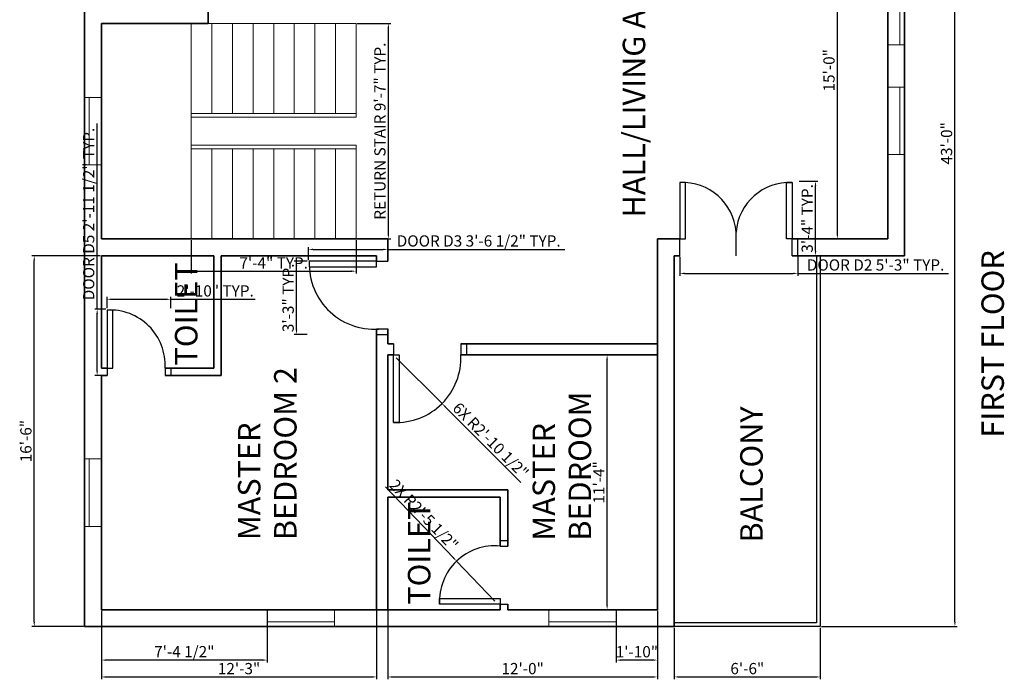
# Model space of a CAD drawing. Units: inches. Extents: x 2641 to 3210, y 2696 to 4064.
# Tile 3 of 4: x 2645 to 3171, y 3425 to 3777. Entities that reach past the tile are written whole.
import ezdxf

# ---------------------------------------------------------------- set-up
doc = ezdxf.new("R2010")
doc.units = ezdxf.units.IN
for name, color, linetype, lineweight in [('A-ANNO-DIMS', 2, 'Continuous', 18), ('A-ANNO-TEXT', 7, 'Continuous', 25), ('A-AREA-IDEN', 7, 'Continuous', 18), ('A-DOOR', 3, 'Continuous', 25), ('A-FLOR-RAIL', 8, 'Continuous', 25), ('A-FLOR-STRS', 7, 'Continuous', 18), ('A-GLAZ', 4, 'Continuous', 18), ('A-WALL', 7, 'Continuous', 35)]:
    doc.layers.add(name, color=color, linetype=linetype, lineweight=lineweight)
doc.styles.get("Standard").update_dxf_attribs({"font": 'arial.ttf'})
doc.dimstyles.new('ISO-25', dxfattribs={"dimtxt": 6, "dimasz": 2.5, "dimexe": 1.25, "dimexo": 0.625, "dimtad": 1, "dimdec": 1, "dimlunit": 3, "dimtxsty": 'Standard', "dimcen": 2.5, "dimadec": 0, "dimazin": 0, "dimtfac": 1, "dimtdec": 1, "dimtmove": 0, "dimatfit": 3, "dimfxl": 1, "dimarcsym": 0})

# ---------------------------------------------------------------- blocks, each defined once
blk = doc.blocks.new('DOOR-36-INT')
for p, q in [((0, 42.03), (0, 36.03)), ((36, 42.03), (36, 36.03)), ((39, 42.03), (39, 36.03))]:
    blk.add_line(p, q)
blk.add_lwpolyline([(0, 36.03), (3, 36.03), (3, 0.03), (0, 0.03)], close=True)
blk.add_arc((1.5, 34.53), 34.53, 267.5104, 2.4896)
blk = doc.blocks.new('DOOR-60-PAIR')
for p, q in [((30, 0), (30, 12.64)), ((0, 0), (0, 9)), ((60, 0), (60, 9)), ((63, 0), (63, 9))]:
    blk.add_line(p, q)
for points in [[(0, 9), (3, 9), (3, 39), (0, 39)], [(60, 9), (57, 9), (57, 39), (60, 39)]]:
    blk.add_lwpolyline(points, close=True)
for centre, start, end in [((1.5, 10.46), 4.3856, 93.0081), ((58.5, 10.46), 86.9919, 175.6144)]:
    blk.add_arc(centre, 28.58, start, end)
blk = doc.blocks.new('DOOR-36-BEDROOM')
for p, q in [((36.03, 39), (42.03, 39)), ((36.03, 3), (42.03, 3)), ((36.03, 0), (42.03, 0))]:
    blk.add_line(p, q)
blk.add_lwpolyline([(36.03, 39), (0.03, 39), (0.03, 36), (36.03, 36)], close=True)
blk.add_arc((34.76, 37.5), 34.76, 177.527, 277.0543)
blk = doc.blocks.new('DOOR-BATH-32P4')
for p, q in [((32.44, 34), (36.44, 34)), ((32.44, 31), (36.44, 31)), ((32.44, 0), (36.44, 0))]:
    blk.add_line(p, q)
blk.add_lwpolyline([(32.44, 0), (0.04, 0), (0.04, 3), (32.44, 3)], close=True)
blk.add_arc((29.63, 1.5), 29.63, 84.5685, 182.9015)
blk = doc.blocks.new('DOOR-31-BATH')
for p, q in [((0, 4), (0, 0)), ((31, 4), (31, 0)), ((34, 4), (34, 0))]:
    blk.add_line(p, q)
blk.add_lwpolyline([(0, 4), (3, 4), (3, 35), (0, 35)], close=True)
blk.add_arc((1.5, 5.5), 29.54, 357.0892, 92.9108)
blk = doc.blocks.new('WIN-36x9')
blk.add_line((6.5, 36), (6.5, 0))
blk.add_lwpolyline([(9, 36), (0, 36), (0, 0), (9, 0)], close=True)
blk = doc.blocks.new('STAIR-RETURN-FLIGHTS')
for p, q in [((0, 0), (0, 115)), ((88, 115), (9, 115)), ((11, 67), (11, 115)), ((22, 67), (22, 115)), ((33, 67), (33, 115)), ((44, 67), (44, 115)), ((55, 67), (55, 115)), ((66, 67), (66, 115)), ((77, 67), (77, 115)), ((88, 67), (88, 115)), ((88, 67), (0, 67)), ((88, 65), (0, 65)), ((88, 65), (88, 67)), ((88, 50), (0, 50)), ((88, 48), (0, 48)), ((11, 0), (11, 48)), ((22, 0), (22, 48)), ((33, 0), (33, 48)), ((44, 0), (44, 48)), ((55, 0), (55, 48)), ((66, 0), (66, 48)), ((77, 0), (77, 48)), ((88, 48), (88, 50)), ((88, 0), (88, 48))]:
    blk.add_line(p, q)
blk = doc.blocks.new('*D35')
at = {"layer": 'A-ANNO-DIMS', "color": 0, "lineweight": -2, "transparency": 16777216}
for p, q in [((2997.63, 3650.77), (2997.63, 3640.69)), ((3060.63, 3650.77), (3060.63, 3640.69)), ((3000.13, 3641.94), (3058.13, 3641.94)), ((3060.63, 3641.94), (3141.17, 3641.94))]:
    blk.add_line(p, q, dxfattribs=at)
at = {"layer": 'A-ANNO-DIMS', "color": 0, "transparency": 16777216}
for points in [[(3000.13, 3642.36), (3000.13, 3641.52), (2997.63, 3641.94)], [(3058.13, 3642.36), (3058.13, 3641.52), (3060.63, 3641.94)]]:
    blk.add_solid(points, dxfattribs=at)
at = {"layer": 'Defpoints', "color": 0, "transparency": 16777216}
for p in [(2997.63, 3651.39), (3060.63, 3651.39), (3060.63, 3641.94)]:
    blk.add_point(p, dxfattribs=at)
at = {"layer": 'A-ANNO-DIMS', "color": 0, "transparency": 16777216, "insert": (3102.15, 3645.67), "char_height": 6, "attachment_point": 5}
blk.add_mtext('DOOR D2 5\'-3" TYP.', dxfattribs=at)
blk = doc.blocks.new('*D36')
at = {"layer": 'A-ANNO-DIMS', "color": 0, "lineweight": -2, "transparency": 16777216}
for p, q in [((3061.25, 3691.2), (3071.33, 3691.2)), ((3070.08, 3653.89), (3070.08, 3688.7)), ((3061.25, 3651.39), (3071.33, 3651.39))]:
    blk.add_line(p, q, dxfattribs=at)
at = {"layer": 'A-ANNO-DIMS', "color": 0, "transparency": 16777216}
for points in [[(3069.66, 3688.7), (3070.49, 3688.7), (3070.08, 3691.2)], [(3069.66, 3653.89), (3070.49, 3653.89), (3070.08, 3651.39)]]:
    blk.add_solid(points, dxfattribs=at)
at = {"layer": 'Defpoints', "color": 0, "transparency": 16777216}
for p in [(3060.63, 3691.2), (3070.08, 3691.2), (3060.63, 3651.39)]:
    blk.add_point(p, dxfattribs=at)
at = {"layer": 'A-ANNO-DIMS', "color": 0, "transparency": 16777216, "insert": (3066.39, 3671.3), "char_height": 6, "attachment_point": 5, "rotation": 90}
blk.add_mtext('3\'-4" TYP.', dxfattribs=at)
blk = doc.blocks.new('*D37')
at = {"layer": 'A-ANNO-DIMS', "color": 0, "lineweight": -2, "transparency": 16777216}
for p, q in [((2799.18, 3649.02), (2799.18, 3656.01)), ((2841.63, 3649.02), (2841.63, 3656.01)), ((2801.68, 3654.76), (2839.13, 3654.76)), ((2841.63, 3654.76), (2936.15, 3654.76))]:
    blk.add_line(p, q, dxfattribs=at)
at = {"layer": 'A-ANNO-DIMS', "color": 0, "transparency": 16777216}
for points in [[(2801.68, 3655.17), (2801.68, 3654.34), (2799.18, 3654.76)], [(2839.13, 3655.17), (2839.13, 3654.34), (2841.63, 3654.76)]]:
    blk.add_solid(points, dxfattribs=at)
at = {"layer": 'Defpoints', "color": 0, "transparency": 16777216}
for p in [(2841.63, 3654.76), (2799.18, 3648.39), (2841.63, 3648.39)]:
    blk.add_point(p, dxfattribs=at)
at = {"layer": 'A-ANNO-DIMS', "color": 0, "transparency": 16777216, "insert": (2890.14, 3658.49), "char_height": 6, "attachment_point": 5}
blk.add_mtext('DOOR D3 3\'-6 1/2" TYP.', dxfattribs=at)
blk = doc.blocks.new('*D38')
at = {"layer": 'A-ANNO-DIMS', "color": 0, "lineweight": -2, "transparency": 16777216}
for p, q in [((2798.56, 3648.39), (2791.57, 3648.39)), ((2792.82, 3611.89), (2792.82, 3645.89)), ((2798.56, 3609.39), (2791.57, 3609.39))]:
    blk.add_line(p, q, dxfattribs=at)
at = {"layer": 'A-ANNO-DIMS', "color": 0, "transparency": 16777216}
for points in [[(2792.4, 3645.89), (2793.24, 3645.89), (2792.82, 3648.39)], [(2792.4, 3611.89), (2793.24, 3611.89), (2792.82, 3609.39)]]:
    blk.add_solid(points, dxfattribs=at)
at = {"layer": 'Defpoints', "color": 0, "transparency": 16777216}
for p in [(2792.82, 3648.39), (2799.18, 3648.39), (2799.18, 3609.39)]:
    blk.add_point(p, dxfattribs=at)
at = {"layer": 'A-ANNO-DIMS', "color": 0, "transparency": 16777216, "insert": (2789.13, 3628.89), "char_height": 6, "attachment_point": 5, "rotation": 90}
blk.add_mtext('3\'-3" TYP.', dxfattribs=at)
blk = doc.blocks.new('*D41')
at = {"layer": 'A-ANNO-DIMS', "color": 0, "lineweight": -2, "transparency": 16777216}
for p, q in [((2686.31, 3622.81), (2686.31, 3722)), ((2691, 3622.81), (2685.06, 3622.81)), ((2686.31, 3589.89), (2686.31, 3620.31)), ((2691, 3587.39), (2685.06, 3587.39))]:
    blk.add_line(p, q, dxfattribs=at)
at = {"layer": 'A-ANNO-DIMS', "color": 0, "transparency": 16777216}
for points in [[(2685.9, 3620.31), (2686.73, 3620.31), (2686.31, 3622.81)], [(2685.9, 3589.89), (2686.73, 3589.89), (2686.31, 3587.39)]]:
    blk.add_solid(points, dxfattribs=at)
at = {"layer": 'Defpoints', "color": 0, "transparency": 16777216}
for p in [(2686.31, 3622.81), (2691.63, 3622.81), (2691.63, 3587.39)]:
    blk.add_point(p, dxfattribs=at)
at = {"layer": 'A-ANNO-DIMS', "color": 0, "transparency": 16777216, "insert": (2682.58, 3673.66), "char_height": 6, "attachment_point": 5, "rotation": 90}
blk.add_mtext('DOOR D5 2\'-11 1/2" TYP.', dxfattribs=at)
blk = doc.blocks.new('*D42')
at = {"layer": 'A-ANNO-DIMS', "color": 0, "lineweight": -2, "transparency": 16777216}
for p, q in [((2691.63, 3623.44), (2691.63, 3629.38)), ((2725.63, 3623.44), (2725.63, 3629.38)), ((2694.13, 3628.13), (2723.13, 3628.13)), ((2725.63, 3628.13), (2770.71, 3628.13))]:
    blk.add_line(p, q, dxfattribs=at)
at = {"layer": 'A-ANNO-DIMS', "color": 0, "transparency": 16777216}
for points in [[(2694.13, 3628.54), (2694.13, 3627.71), (2691.63, 3628.13)], [(2723.13, 3628.54), (2723.13, 3627.71), (2725.63, 3628.13)]]:
    blk.add_solid(points, dxfattribs=at)
at = {"layer": 'Defpoints', "color": 0, "transparency": 16777216}
for p in [(2725.63, 3628.13), (2691.63, 3622.81), (2725.63, 3622.81)]:
    blk.add_point(p, dxfattribs=at)
at = {"layer": 'A-ANNO-DIMS', "color": 0, "transparency": 16777216, "insert": (2749.42, 3631.82), "char_height": 6, "attachment_point": 5}
blk.add_mtext('2\'-10" TYP.', dxfattribs=at)
blk = doc.blocks.new('*D49')
at = {"layer": 'A-ANNO-DIMS', "color": 0, "lineweight": -2, "transparency": 16777216}
for p, q in [((2825.25, 3775.39), (2843.13, 3775.39)), ((2841.88, 3662.89), (2841.88, 3772.89)), ((2825.25, 3660.39), (2843.13, 3660.39))]:
    blk.add_line(p, q, dxfattribs=at)
at = {"layer": 'A-ANNO-DIMS', "color": 0, "transparency": 16777216}
for points in [[(2841.46, 3772.89), (2842.29, 3772.89), (2841.88, 3775.39)], [(2841.46, 3662.89), (2842.29, 3662.89), (2841.88, 3660.39)]]:
    blk.add_solid(points, dxfattribs=at)
at = {"layer": 'Defpoints', "color": 0, "transparency": 16777216}
for p in [(2824.63, 3775.39), (2841.88, 3775.39), (2824.63, 3660.39)]:
    blk.add_point(p, dxfattribs=at)
at = {"layer": 'A-ANNO-DIMS', "color": 0, "transparency": 16777216, "insert": (2838.15, 3717.89), "char_height": 6, "attachment_point": 5, "rotation": 90}
blk.add_mtext('RETURN STAIR 9\'-7" TYP.', dxfattribs=at)
blk = doc.blocks.new('*D50')
at = {"layer": 'A-ANNO-DIMS', "color": 0, "lineweight": -2, "transparency": 16777216}
for p, q in [((2736.63, 3659.77), (2736.63, 3641.89)), ((2824.63, 3659.77), (2824.63, 3641.89)), ((2739.13, 3643.14), (2822.13, 3643.14))]:
    blk.add_line(p, q, dxfattribs=at)
at = {"layer": 'A-ANNO-DIMS', "color": 0, "transparency": 16777216}
for points in [[(2739.13, 3643.56), (2739.13, 3642.72), (2736.63, 3643.14)], [(2822.13, 3643.56), (2822.13, 3642.72), (2824.63, 3643.14)]]:
    blk.add_solid(points, dxfattribs=at)
at = {"layer": 'Defpoints', "color": 0, "transparency": 16777216}
for p in [(2736.63, 3660.39), (2824.63, 3660.39), (2824.63, 3643.14)]:
    blk.add_point(p, dxfattribs=at)
at = {"layer": 'A-ANNO-DIMS', "color": 0, "transparency": 16777216, "insert": (2780.63, 3646.77), "char_height": 6, "attachment_point": 5}
blk.add_mtext('7\'-4" TYP.', dxfattribs=at)
blk = doc.blocks.new('*D67')
at = {"layer": 'A-ANNO-DIMS', "color": 0, "lineweight": -2, "transparency": 16777216}
for p, q in [((3118.25, 3969.39), (3145.78, 3969.39)), ((3144.53, 3455.89), (3144.53, 3966.89)), ((3073.25, 3453.39), (3145.78, 3453.39))]:
    blk.add_line(p, q, dxfattribs=at)
at = {"layer": 'A-ANNO-DIMS', "color": 0, "transparency": 16777216}
for points in [[(3144.11, 3966.89), (3144.94, 3966.89), (3144.53, 3969.39)], [(3144.11, 3455.89), (3144.94, 3455.89), (3144.53, 3453.39)]]:
    blk.add_solid(points, dxfattribs=at)
at = {"layer": 'Defpoints', "color": 0, "transparency": 16777216}
for p in [(3117.63, 3969.39), (3144.53, 3969.39), (3072.63, 3453.39)]:
    blk.add_point(p, dxfattribs=at)
at = {"layer": 'A-ANNO-DIMS', "color": 0, "transparency": 16777216, "insert": (3140.84, 3711.39), "char_height": 6, "attachment_point": 5, "rotation": 90}
blk.add_mtext('43\'-0"', dxfattribs=at)
blk = doc.blocks.new('*D68')
at = {"layer": 'A-ANNO-DIMS', "color": 0, "lineweight": -2, "transparency": 16777216}
for p, q in [((2688.63, 3461.77), (2688.63, 3425.24)), ((2835.63, 3461.77), (2835.63, 3425.24)), ((2691.13, 3426.49), (2833.13, 3426.49))]:
    blk.add_line(p, q, dxfattribs=at)
at = {"layer": 'A-ANNO-DIMS', "color": 0, "transparency": 16777216}
for points in [[(2691.13, 3426.91), (2691.13, 3426.07), (2688.63, 3426.49)], [(2833.13, 3426.91), (2833.13, 3426.07), (2835.63, 3426.49)]]:
    blk.add_solid(points, dxfattribs=at)
at = {"layer": 'Defpoints', "color": 0, "transparency": 16777216}
for p in [(2688.63, 3462.39), (2835.63, 3462.39), (2835.63, 3426.49)]:
    blk.add_point(p, dxfattribs=at)
at = {"layer": 'A-ANNO-DIMS', "color": 0, "transparency": 16777216, "insert": (2762.13, 3430.18), "char_height": 6, "attachment_point": 5}
blk.add_mtext('12\'-3"', dxfattribs=at)
blk = doc.blocks.new('*D69')
at = {"layer": 'A-ANNO-DIMS', "color": 0, "lineweight": -2, "transparency": 16777216}
for p, q in [((2841.63, 3461.77), (2841.63, 3425.24)), ((2985.63, 3461.77), (2985.63, 3425.24)), ((2844.13, 3426.49), (2983.13, 3426.49))]:
    blk.add_line(p, q, dxfattribs=at)
at = {"layer": 'A-ANNO-DIMS', "color": 0, "transparency": 16777216}
for points in [[(2844.13, 3426.91), (2844.13, 3426.07), (2841.63, 3426.49)], [(2983.13, 3426.91), (2983.13, 3426.07), (2985.63, 3426.49)]]:
    blk.add_solid(points, dxfattribs=at)
at = {"layer": 'Defpoints', "color": 0, "transparency": 16777216}
for p in [(2841.63, 3462.39), (2985.63, 3462.39), (2985.63, 3426.49)]:
    blk.add_point(p, dxfattribs=at)
at = {"layer": 'A-ANNO-DIMS', "color": 0, "transparency": 16777216, "insert": (2913.63, 3430.18), "char_height": 6, "attachment_point": 5}
blk.add_mtext('12\'-0"', dxfattribs=at)
blk = doc.blocks.new('*D70')
at = {"layer": 'A-ANNO-DIMS', "color": 0, "lineweight": -2, "transparency": 16777216}
for p, q in [((2688, 3651.39), (2651.48, 3651.39)), ((2652.73, 3455.89), (2652.73, 3648.89)), ((2679, 3453.39), (2651.48, 3453.39))]:
    blk.add_line(p, q, dxfattribs=at)
at = {"layer": 'A-ANNO-DIMS', "color": 0, "transparency": 16777216}
for points in [[(2652.31, 3648.89), (2653.14, 3648.89), (2652.73, 3651.39)], [(2652.31, 3455.89), (2653.14, 3455.89), (2652.73, 3453.39)]]:
    blk.add_solid(points, dxfattribs=at)
at = {"layer": 'Defpoints', "color": 0, "transparency": 16777216}
for p in [(2652.73, 3651.39), (2688.63, 3651.39), (2679.63, 3453.39)]:
    blk.add_point(p, dxfattribs=at)
at = {"layer": 'A-ANNO-DIMS', "color": 0, "transparency": 16777216, "insert": (2649.04, 3552.39), "char_height": 6, "attachment_point": 5, "rotation": 90}
blk.add_mtext('16\'-6"', dxfattribs=at)
blk = doc.blocks.new('*D71')
at = {"layer": 'A-ANNO-DIMS', "color": 0, "lineweight": -2, "transparency": 16777216}
for p, q in [((2994.63, 3452.77), (2994.63, 3425.24)), ((3072.63, 3452.77), (3072.63, 3425.24)), ((2997.13, 3426.49), (3070.13, 3426.49))]:
    blk.add_line(p, q, dxfattribs=at)
at = {"layer": 'A-ANNO-DIMS', "color": 0, "transparency": 16777216}
for points in [[(2997.13, 3426.91), (2997.13, 3426.07), (2994.63, 3426.49)], [(3070.13, 3426.91), (3070.13, 3426.07), (3072.63, 3426.49)]]:
    blk.add_solid(points, dxfattribs=at)
at = {"layer": 'Defpoints', "color": 0, "transparency": 16777216}
for p in [(2994.63, 3453.39), (3072.63, 3453.39), (3072.63, 3426.49)]:
    blk.add_point(p, dxfattribs=at)
at = {"layer": 'A-ANNO-DIMS', "color": 0, "transparency": 16777216, "insert": (3033.63, 3430.18), "char_height": 6, "attachment_point": 5}
blk.add_mtext('6\'-6"', dxfattribs=at)
blk = doc.blocks.new('*D79')
at = {"layer": 'A-ANNO-DIMS', "color": 0, "lineweight": -2, "transparency": 16777216}
for p, q in [((2985, 3598.39), (2957.48, 3598.39)), ((2958.73, 3464.89), (2958.73, 3595.89)), ((2985, 3462.39), (2957.48, 3462.39))]:
    blk.add_line(p, q, dxfattribs=at)
at = {"layer": 'A-ANNO-DIMS', "color": 0, "transparency": 16777216}
for points in [[(2958.31, 3595.89), (2959.14, 3595.89), (2958.73, 3598.39)], [(2958.31, 3464.89), (2959.14, 3464.89), (2958.73, 3462.39)]]:
    blk.add_solid(points, dxfattribs=at)
at = {"layer": 'Defpoints', "color": 0, "transparency": 16777216}
for p in [(2958.73, 3598.39), (2985.63, 3598.39), (2985.63, 3462.39)]:
    blk.add_point(p, dxfattribs=at)
at = {"layer": 'A-ANNO-DIMS', "color": 0, "transparency": 16777216, "insert": (2955.09, 3530.39), "char_height": 6, "attachment_point": 5, "rotation": 90}
blk.add_mtext('11\'-4"', dxfattribs=at)
blk = doc.blocks.new('*D80')
at = {"layer": 'A-ANNO-DIMS', "color": 0, "lineweight": -2, "transparency": 16777216}
for p, q in [((3108, 3840.39), (3080.48, 3840.39)), ((3081.73, 3662.89), (3081.73, 3837.89)), ((3108, 3660.39), (3080.48, 3660.39))]:
    blk.add_line(p, q, dxfattribs=at)
at = {"layer": 'A-ANNO-DIMS', "color": 0, "transparency": 16777216}
for points in [[(3081.31, 3837.89), (3082.14, 3837.89), (3081.73, 3840.39)], [(3081.31, 3662.89), (3082.14, 3662.89), (3081.73, 3660.39)]]:
    blk.add_solid(points, dxfattribs=at)
at = {"layer": 'Defpoints', "color": 0, "transparency": 16777216}
for p in [(3081.73, 3840.39), (3108.63, 3840.39), (3108.63, 3660.39)]:
    blk.add_point(p, dxfattribs=at)
at = {"layer": 'A-ANNO-DIMS', "color": 0, "transparency": 16777216, "insert": (3078.04, 3750.39), "char_height": 6, "attachment_point": 5, "rotation": 90}
blk.add_mtext('15\'-0"', dxfattribs=at)
blk = doc.blocks.new('*D83')
at = {"layer": 'A-ANNO-DIMS', "color": 0, "lineweight": -2, "transparency": 16777216}
for p, q in [((2688.63, 3461.77), (2688.63, 3434.24)), ((2777.13, 3461.77), (2777.13, 3434.24)), ((2774.63, 3435.49), (2691.13, 3435.49))]:
    blk.add_line(p, q, dxfattribs=at)
at = {"layer": 'A-ANNO-DIMS', "color": 0, "transparency": 16777216}
for points in [[(2691.13, 3435.91), (2691.13, 3435.07), (2688.63, 3435.49)], [(2774.63, 3435.91), (2774.63, 3435.07), (2777.13, 3435.49)]]:
    blk.add_solid(points, dxfattribs=at)
at = {"layer": 'Defpoints', "color": 0, "transparency": 16777216}
for p in [(2688.63, 3462.39), (2777.13, 3462.39), (2688.63, 3435.49)]:
    blk.add_point(p, dxfattribs=at)
at = {"layer": 'A-ANNO-DIMS', "color": 0, "transparency": 16777216, "insert": (2732.88, 3439.22), "char_height": 6, "attachment_point": 5}
blk.add_mtext('7\'-4 1/2"', dxfattribs=at)
blk = doc.blocks.new('*D84')
at = {"layer": 'A-ANNO-DIMS', "color": 0, "lineweight": -2, "transparency": 16777216}
for p, q in [((2963.63, 3461.77), (2963.63, 3434.24)), ((2985.63, 3461.77), (2985.63, 3434.24)), ((2983.13, 3435.49), (2966.13, 3435.49))]:
    blk.add_line(p, q, dxfattribs=at)
at = {"layer": 'A-ANNO-DIMS', "color": 0, "transparency": 16777216}
for points in [[(2966.13, 3435.91), (2966.13, 3435.07), (2963.63, 3435.49)], [(2983.13, 3435.91), (2983.13, 3435.07), (2985.63, 3435.49)]]:
    blk.add_solid(points, dxfattribs=at)
at = {"layer": 'Defpoints', "color": 0, "transparency": 16777216}
for p in [(2963.63, 3462.39), (2985.63, 3462.39), (2963.63, 3435.49)]:
    blk.add_point(p, dxfattribs=at)
at = {"layer": 'A-ANNO-DIMS', "color": 0, "transparency": 16777216, "insert": (2974.63, 3439.18), "char_height": 6, "attachment_point": 5}
blk.add_mtext('1\'-10"', dxfattribs=at)
blk = doc.blocks.new('*D86')
at = {"layer": 'A-ANNO-DIMS', "color": 0, "lineweight": -2, "transparency": 16777216}
for p, q in [((2846.13, 3596.89), (2870.54, 3572.47)), ((2912.62, 3530.39), (2872.31, 3570.7))]:
    blk.add_line(p, q, dxfattribs=at)
at = {"layer": 'A-ANNO-DIMS', "color": 0, "transparency": 16777216}
blk.add_solid([(2872.61, 3571), (2872.02, 3570.41), (2870.54, 3572.47)], dxfattribs=at)
at = {"layer": 'Defpoints', "color": 0, "transparency": 16777216}
for p in [(2846.13, 3596.89), (2870.54, 3572.47)]:
    blk.add_point(p, dxfattribs=at)
at = {"layer": 'A-ANNO-DIMS', "color": 0, "transparency": 16777216, "insert": (2895.99, 3552.3), "char_height": 6, "attachment_point": 5, "rotation": 315}
blk.add_mtext('6X R2\'-10 1/2"', dxfattribs=at)
blk = doc.blocks.new('*D88')
at = {"layer": 'A-ANNO-DIMS', "color": 0, "lineweight": -2, "transparency": 16777216}
for p, q in [((2840.37, 3527.98), (2876.61, 3490.11)), ((2898.82, 3466.89), (2878.33, 3488.3))]:
    blk.add_line(p, q, dxfattribs=at)
at = {"layer": 'A-ANNO-DIMS', "color": 0, "transparency": 16777216}
blk.add_solid([(2876.91, 3490.4), (2876.31, 3489.82), (2878.33, 3488.3)], dxfattribs=at)
at = {"layer": 'Defpoints', "color": 0, "transparency": 16777216}
for p in [(2878.33, 3488.3), (2898.82, 3466.89)]:
    blk.add_point(p, dxfattribs=at)
at = {"layer": 'A-ANNO-DIMS', "color": 0, "transparency": 16777216, "insert": (2860.32, 3512.52), "char_height": 6, "attachment_point": 5, "rotation": 313.7353}
blk.add_mtext('2X R2\'-5 1/2"', dxfattribs=at)

msp = doc.modelspace()

# ---------------------------------------------------------------- linework, layer by layer
at = {"layer": 'A-FLOR-RAIL'}
for p, q in [((3060.63, 3651.39), (3072.63, 3651.39)), ((3070.63, 3651.39), (3070.63, 3455.39)), ((3072.63, 3651.39), (3072.63, 3453.39)), ((3070.63, 3455.39), (2994.63, 3455.39)), ((3072.63, 3453.39), (2994.63, 3453.39))]:
    msp.add_line(p, q, dxfattribs=at)
at = {"layer": 'A-WALL'}
for p, q in [((2679.63, 3453.39), (2679.63, 3969.39)), ((3108.63, 3840.39), (3108.63, 3723.39)), ((2745.63, 3775.39), (2745.63, 3782.39)), ((2688.63, 3660.39), (2688.63, 3775.39)), ((2688.63, 3775.39), (2745.63, 3775.39)), ((3108.63, 3723.39), (3108.63, 3660.39)), ((2841.63, 3660.39), (2688.63, 3660.39)), ((2841.63, 3660.39), (2841.63, 3648.39)), ((2997.63, 3660.39), (2985.63, 3660.39)), ((2985.63, 3660.39), (2985.63, 3612.39)), ((3108.63, 3660.39), (3057.63, 3660.39)), ((2688.63, 3591.39), (2688.63, 3651.39)), ((2748.63, 3651.39), (2688.63, 3651.39)), ((2748.63, 3591.39), (2748.63, 3651.39)), ((2752.63, 3587.39), (2752.63, 3651.39)), ((2835.63, 3651.39), (2752.63, 3651.39)), ((2835.63, 3651.39), (2835.63, 3648.39)), ((2835.63, 3651.39), (2835.63, 3648.39)), ((2997.63, 3651.39), (2994.63, 3651.39)), ((2994.63, 3651.39), (2994.63, 3453.39)), ((2994.63, 3651.39), (2997.63, 3651.39)), ((3117.63, 3651.39), (3057.63, 3651.39)), ((2835.63, 3612.39), (2835.63, 3462.39)), ((2841.63, 3612.39), (2841.63, 3604.39)), ((2985.63, 3606.39), (2985.63, 3612.39)), ((2841.63, 3604.39), (2844.63, 3604.39)), ((2841.63, 3604.39), (2844.63, 3604.39)), ((2880.63, 3604.39), (2985.63, 3604.39)), ((2985.63, 3606.39), (2985.63, 3462.39)), ((2841.63, 3598.39), (2841.63, 3526.39)), ((2841.63, 3598.39), (2844.63, 3598.39)), ((2880.63, 3598.39), (2985.63, 3598.39)), ((2691.63, 3591.39), (2688.63, 3591.39)), ((2688.63, 3591.39), (2691.63, 3591.39)), ((2688.63, 3462.39), (2688.63, 3587.39)), ((2691.63, 3587.39), (2688.63, 3587.39)), ((2748.63, 3591.39), (2722.63, 3591.39)), ((2752.63, 3587.39), (2722.63, 3587.39)), ((2905.63, 3526.39), (2841.63, 3526.39)), ((2905.63, 3526.39), (2905.63, 3496.39)), ((2841.63, 3522.39), (2841.63, 3462.39)), ((2901.63, 3522.39), (2841.63, 3522.39)), ((2901.63, 3522.39), (2901.63, 3496.39)), ((2901.63, 3462.39), (2688.63, 3462.39)), ((2901.63, 3465.39), (2901.63, 3462.39)), ((2901.63, 3462.39), (2901.63, 3465.39)), ((2905.63, 3465.39), (2905.63, 3462.39)), ((2985.63, 3462.39), (2905.63, 3462.39))]:
    msp.add_line(p, q, dxfattribs=at)
for points in [[(3072.63, 3969.39), (3117.63, 3969.39), (3117.63, 3723.39)], [(3117.63, 3723.39), (3117.63, 3651.39)], [(2994.63, 3453.39), (2679.63, 3453.39)]]:
    msp.add_lwpolyline(points, dxfattribs=at)

# ---------------------------------------------------------------- block references
at = {"layer": 'A-DOOR'}
for name, p in [('DOOR-60-PAIR', (2997.63, 3651.39)), ('DOOR-36-BEDROOM', (2799.6, 3609.39)), ('DOOR-31-BATH', (2691.63, 3587.39)), ('DOOR-36-INT', (2844.63, 3562.36)), ('DOOR-BATH-32P4', (2869.19, 3465.39))]:
    msp.add_blockref(name, p, dxfattribs=at)
at = {"layer": 'A-FLOR-STRS'}
msp.add_blockref('STAIR-RETURN-FLIGHTS', (2736.63, 3660.39), dxfattribs=at)
at = {"layer": 'A-GLAZ'}
for p in [(3108.63, 3763.89), (3108.63, 3705.39)]:
    msp.add_blockref('WIN-36x9', p, dxfattribs=at)
for p, rotation in [((2688.63, 3735.89), 180), ((2688.63, 3542.89), 180), ((2777.13, 3462.39), 269.9999999999978), ((2927.63, 3462.39), 269.9999999999982)]:
    msp.add_blockref('WIN-36x9', p, dxfattribs=dict(at, rotation=rotation))

# ---------------------------------------------------------------- texts
at = {"layer": 'A-ANNO-TEXT'}
msp.add_text('FIRST FLOOR', height=12, rotation=90, dxfattribs=at).set_placement((3170.7, 3554.27))
at = {"layer": 'A-AREA-IDEN'}
for s, p in [('HALL/LIVING AREA', (2979.08, 3671.82)), ('TOILET', (2739.91, 3592.76)), ('BEDROOM 2', (2792.84, 3499.51)), ('BEDROOM', (2950.21, 3499.24)), ('BALCONY', (3041.83, 3498.24)), ('MASTER', (2773.56, 3499.51)), ('MASTER', (2930.93, 3499.24)), ('TOILET', (2864.32, 3465.03))]:
    msp.add_text(s, height=12, rotation=90, dxfattribs=at).set_placement(p)

# ---------------------------------------------------------------- dimensions: what is measured, and where the dimension line sits
at = {"layer": 'A-ANNO-DIMS'}
for base, p1, p2, angle, picture, middle in [((3144.53, 3969.39), (3072.63, 3453.39), (3117.63, 3969.39), 90, '*D67', (3140.84, 3711.39)), ((3081.73, 3840.39), (3108.63, 3660.39), (3108.63, 3840.39), 90, '*D80', (3078.04, 3750.39)), ((2652.73, 3651.39), (2679.63, 3453.39), (2688.63, 3651.39), 90, '*D70', (2649.04, 3552.39)), ((2958.73, 3598.39), (2985.63, 3462.39), (2985.63, 3598.39), 90, '*D79', (2955.09, 3530.39)), ((2688.63, 3435.49), (2777.13, 3462.39), (2688.63, 3462.39), 180, '*D83', (2732.88, 3439.22)), ((2963.63, 3435.49), (2985.63, 3462.39), (2963.63, 3462.39), 180, '*D84', (2974.63, 3439.18))]:
    dim = msp.add_linear_dim(base=base, p1=p1, p2=p2, angle=angle, dimstyle='ISO-25', override={"dimdec": 1, "dimlfac": 1, "dimrnd": 0, "dimzin": 1, "dimdsep": 46, "dimlunit": 4, "dimfrac": 2}, dxfattribs=at)
    dim.commit()
    dim.dimension.update_dxf_attribs({"geometry": picture, "text_midpoint": middle})
for base, p1, p2, text, picture, middle in [((2841.88, 3775.39), (2824.63, 3660.39), (2824.63, 3775.39), 'RETURN STAIR <> TYP.', '*D49', (2838.15, 3717.89)), ((2686.31, 3622.81), (2691.63, 3587.39), (2691.63, 3622.81), 'DOOR D5 <> TYP.', '*D41', (2682.58, 3673.66)), ((3070.08, 3691.2), (3060.63, 3651.39), (3060.63, 3691.2), '<> TYP.', '*D36', (3066.39, 3671.3)), ((2792.82, 3648.39), (2799.18, 3609.39), (2799.18, 3648.39), '<> TYP.', '*D38', (2789.13, 3628.89))]:
    dim = msp.add_linear_dim(base=base, p1=p1, p2=p2, angle=90, text=text, dimstyle='ISO-25', override={"dimdec": 1, "dimlfac": 1, "dimrnd": 0, "dimzin": 1, "dimdsep": 46, "dimlunit": 4, "dimfrac": 2}, dxfattribs=at)
    dim.commit()
    dim.dimension.update_dxf_attribs({"geometry": picture, "text_midpoint": middle})
for base, p1, p2, text, picture, middle in [((2841.6258, 3654.7563), (2799.1846, 3648.3901), (2841.6258, 3648.3901), 'DOOR D3 <> TYP.', '*D37', (2890.1376, 3658.4877)), ((3060.63, 3641.94), (2997.63, 3651.39), (3060.63, 3651.39), 'DOOR D2 <> TYP.', '*D35', (3102.15, 3645.67)), ((2824.63, 3643.14), (2736.63, 3660.39), (2824.63, 3660.39), '<> TYP.', '*D50', (2780.63, 3646.77)), ((2725.63, 3628.13), (2691.63, 3622.81), (2725.63, 3622.81), '<> TYP.', '*D42', (2749.42, 3631.82))]:
    dim = msp.add_linear_dim(base=base, p1=p1, p2=p2, text=text, dimstyle='ISO-25', override={"dimdec": 1, "dimlfac": 1, "dimrnd": 0, "dimzin": 1, "dimdsep": 46, "dimlunit": 4, "dimfrac": 2}, dxfattribs=at)
    dim.commit()
    dim.dimension.update_dxf_attribs({"geometry": picture, "text_midpoint": middle})
for center, mpoint, text, picture, middle in [((2846.13, 3596.89), (2870.54, 3572.47), '6X <>', '*D86', (2895.99, 3552.3)), ((2898.82, 3466.89), (2878.33, 3488.3), '2X <>', '*D88', (2860.32, 3512.52))]:
    dim = msp.add_radius_dim(center=center, mpoint=mpoint, text=text, dimstyle='ISO-25', override={"dimdec": 1, "dimlfac": 1, "dimrnd": 0, "dimzin": 1, "dimdsep": 46, "dimlunit": 4, "dimfrac": 2}, dxfattribs=at)
    dim.commit()
    dim.dimension.update_dxf_attribs({"geometry": picture, "text_midpoint": middle})
for base, p1, p2, picture, middle in [((2835.63, 3426.49), (2688.63, 3462.39), (2835.63, 3462.39), '*D68', (2762.13, 3430.18)), ((2985.63, 3426.49), (2841.63, 3462.39), (2985.63, 3462.39), '*D69', (2913.63, 3430.18)), ((3072.63, 3426.49), (2994.63, 3453.39), (3072.63, 3453.39), '*D71', (3033.63, 3430.18))]:
    dim = msp.add_linear_dim(base=base, p1=p1, p2=p2, dimstyle='ISO-25', override={"dimdec": 1, "dimlfac": 1, "dimrnd": 0, "dimzin": 1, "dimdsep": 46, "dimlunit": 4, "dimfrac": 2}, dxfattribs=at)
    dim.commit()
    dim.dimension.update_dxf_attribs({"geometry": picture, "text_midpoint": middle})

doc.saveas('drawing.dxf')
